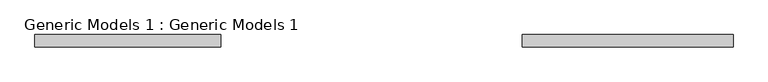
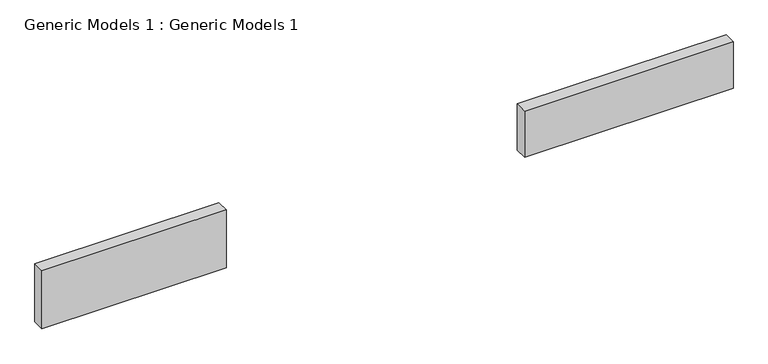
"""IFC4 building model written with IfcOpenShell, lengths in millimetres: proxy geometry, Generic Models 1 : Generic Models 1."""

from ifc_helpers import new_model, si_unit, frame, origin, place, context, project, spatial, polyline, outline, extrude, source, transform, mapped, element, save


def generic_models_1_generic_models_1_74e75cdd(model_context):
    return source(origin(), model_context, "Body", "SweptSolid", [
        extrude(outline(polyline([(-3137.418004, -8964.0383207), (-5423.418004, -8964.0383207), (-5423.418004, -8811.6383207), (-3137.418004, -8811.6383207), (-3137.418004, -8964.0383207)])), frame((0.0, 0.0, 435.8822488), z_axis=(0.0, 0.0, 1.0), x_axis=(1.0, 0.0, 0.0)), (0.0, 0.0, 1.0), 762.0),
        extrude(outline(polyline([(3160.7557588, -8964.0383207), (569.9557588, -8964.0383207), (569.9557588, -8811.6383207), (3160.7557588, -8811.6383207), (3160.7557588, -8964.0383207)])), frame((0.0, 0.0, 588.2822488), z_axis=(0.0, 0.0, 1.0), x_axis=(1.0, 0.0, 0.0)), (0.0, 0.0, 1.0), 609.6),
    ])


if __name__ == "__main__":
    model = new_model("IFC4")
    model_context = context("Model", 3, world=origin())
    ifc_project = project(units=[si_unit("LENGTHUNIT", "METRE", prefix="MILLI")], contexts=[model_context])
    site = spatial("IfcSite", under=ifc_project)
    building = spatial("IfcBuilding", under=site)
    placement = place(None, origin())
    generic_models_1_generic_models_1_shape = generic_models_1_generic_models_1_74e75cdd(model_context)
    element("IfcBuildingElementProxy", 1, Name="Generic Models 1 : Generic Models 1", ObjectType="Generic Models 1 : Generic Models 1", at=placement, inside=building, context=model_context, shape_type="MappedRepresentation", body=[
        mapped(generic_models_1_generic_models_1_shape, transform((0.0, 0.0, 0.0), x_axis=(1.0, 0.0, 0.0), y_axis=(0.0, 1.0, 0.0), z_axis=(0.0, 0.0, 1.0))),
    ])
    save(model, "model.ifc")

# Revit data of these elements
# Element 1 (IfcBuildingElementProxy, "Generic Models 1 : Generic Models 1")
#   Materials on its faces: "Blanket"
# Materials
#   "Blanket": class "System", colour RGB 59 0 1, transparency 0, Cost = 0
